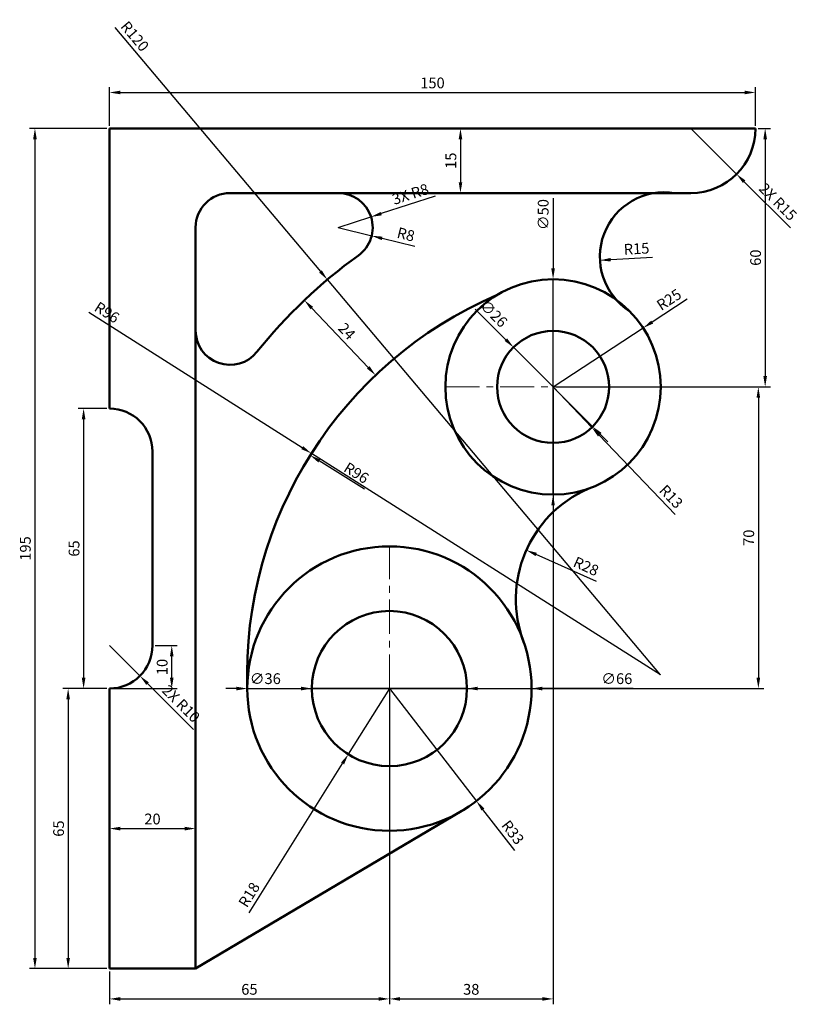
# Model space of a CAD drawing. Units: millimetres. Extents: x 2491 to 2672, y 889 to 1118.
import ezdxf

# ---------------------------------------------------------------- set-up
doc = ezdxf.new("R2010")
doc.units = ezdxf.units.MM
doc.linetypes.add('CENTER', pattern=[50.8, 31.75, -6.35, 6.35, -6.35])
for name, color, linetype, lineweight in [('M-CNTR', 4, 'CENTER', 18), ('M-DIMS', 2, 'Continuous', 25), ('M-OUTL', 7, 'Continuous', 50)]:
    doc.layers.add(name, color=color, linetype=linetype, lineweight=lineweight)
doc.styles.get("Standard").update_dxf_attribs({"font": 'arial.ttf'})
doc.dimstyles.new('ISO-25', dxfattribs={"dimtxt": 2.5, "dimasz": 2.5, "dimexe": 1.25, "dimexo": 0.625, "dimtad": 1, "dimtxsty": 'Standard', "dimcen": 2.5, "dimadec": 0, "dimazin": 0, "dimtfac": 1, "dimtmove": 0, "dimatfit": 3, "dimfxl": 1, "dimarcsym": 0})

# ---------------------------------------------------------------- blocks, each defined once
blk = doc.blocks.new('*D1')
at = {"layer": 'Defpoints', "color": 0, "transparency": 16777216}
for p in [(2511.93, 1092.34), (2494.64, 897.34), (2511.93, 897.34)]:
    blk.add_point(p, dxfattribs=at)
at = {"layer": 'M-DIMS', "color": 0, "lineweight": -2, "transparency": 16777216}
for p, q in [((2511.31, 1092.34), (2493.39, 1092.34)), ((2494.64, 1089.84), (2494.64, 899.84)), ((2511.31, 897.34), (2493.39, 897.34))]:
    blk.add_line(p, q, dxfattribs=at)
at = {"layer": 'M-DIMS', "color": 0, "transparency": 16777216}
for points in [[(2494.22, 1089.84), (2495.06, 1089.84), (2494.64, 1092.34)], [(2494.22, 899.84), (2495.06, 899.84), (2494.64, 897.34)]]:
    blk.add_solid(points, dxfattribs=at)
at = {"layer": 'M-DIMS', "color": 0, "transparency": 16777216, "insert": (2492.74, 994.84), "char_height": 2.5, "attachment_point": 5, "rotation": 90}
blk.add_mtext('195', dxfattribs=at)
blk = doc.blocks.new('*D2')
at = {"layer": 'Defpoints', "color": 0, "transparency": 16777216}
for p in [(2661.93, 1100.67), (2511.93, 1092.34), (2661.93, 1092.34)]:
    blk.add_point(p, dxfattribs=at)
at = {"layer": 'M-DIMS', "color": 0, "lineweight": -2, "transparency": 16777216}
for p, q in [((2511.93, 1092.96), (2511.93, 1101.92)), ((2661.93, 1092.96), (2661.93, 1101.92)), ((2514.43, 1100.67), (2659.43, 1100.67))]:
    blk.add_line(p, q, dxfattribs=at)
at = {"layer": 'M-DIMS', "color": 0, "transparency": 16777216}
for points in [[(2514.43, 1101.09), (2514.43, 1100.26), (2511.93, 1100.67)], [(2659.43, 1101.09), (2659.43, 1100.26), (2661.93, 1100.67)]]:
    blk.add_solid(points, dxfattribs=at)
at = {"layer": 'M-DIMS', "color": 0, "transparency": 16777216, "insert": (2586.93, 1102.57), "char_height": 2.5, "attachment_point": 5}
blk.add_mtext('150', dxfattribs=at)
blk = doc.blocks.new('*D3')
at = {"layer": 'Defpoints', "color": 0, "transparency": 16777216}
for p in [(2586.93, 1092.34), (2586.93, 1077.34), (2593.43, 1077.34)]:
    blk.add_point(p, dxfattribs=at)
at = {"layer": 'M-DIMS', "color": 0, "lineweight": -2, "transparency": 16777216}
for p, q in [((2587.56, 1092.34), (2594.68, 1092.34)), ((2593.43, 1089.84), (2593.43, 1079.84)), ((2587.56, 1077.34), (2594.68, 1077.34))]:
    blk.add_line(p, q, dxfattribs=at)
at = {"layer": 'M-DIMS', "color": 0, "transparency": 16777216}
for points in [[(2593.02, 1089.84), (2593.85, 1089.84), (2593.43, 1092.34)], [(2593.02, 1079.84), (2593.85, 1079.84), (2593.43, 1077.34)]]:
    blk.add_solid(points, dxfattribs=at)
at = {"layer": 'M-DIMS', "color": 0, "transparency": 16777216, "insert": (2591.53, 1084.84), "char_height": 2.5, "attachment_point": 5, "rotation": 90}
blk.add_mtext('15', dxfattribs=at)
blk = doc.blocks.new('*D4')
at = {"layer": 'Defpoints', "color": 0, "transparency": 16777216}
for p in [(2557.19, 1052.45), (2573.73, 1035.06), (2573.73, 1035.06)]:
    blk.add_point(p, dxfattribs=at)
at = {"layer": 'M-DIMS', "color": 0, "lineweight": -2, "transparency": 16777216}
for p, q in [((2557.65, 1052.89), (2558.1, 1053.32)), ((2558.92, 1050.64), (2572.01, 1036.87)), ((2574.18, 1035.49), (2574.64, 1035.92))]:
    blk.add_line(p, q, dxfattribs=at)
at = {"layer": 'M-DIMS', "color": 0, "transparency": 16777216}
for points in [[(2559.22, 1050.93), (2558.61, 1050.36), (2557.19, 1052.45)], [(2572.31, 1037.16), (2571.71, 1036.59), (2573.73, 1035.06)]]:
    blk.add_solid(points, dxfattribs=at)
at = {"layer": 'M-DIMS', "color": 0, "transparency": 16777216, "insert": (2566.82, 1045.05), "char_height": 2.5, "attachment_point": 5, "rotation": 313.5577}
blk.add_mtext('24', dxfattribs=at)
blk = doc.blocks.new('*D5')
at = {"layer": 'Defpoints', "color": 0, "transparency": 16777216}
for p in [(2661.93, 1092.34), (2614.93, 1032.34), (2664.17, 1032.34)]:
    blk.add_point(p, dxfattribs=at)
at = {"layer": 'M-DIMS', "color": 0, "lineweight": -2, "transparency": 16777216}
for p, q in [((2662.56, 1092.34), (2665.42, 1092.34)), ((2664.17, 1089.84), (2664.17, 1034.84)), ((2615.56, 1032.34), (2665.42, 1032.34))]:
    blk.add_line(p, q, dxfattribs=at)
at = {"layer": 'M-DIMS', "color": 0, "transparency": 16777216}
for points in [[(2663.76, 1089.84), (2664.59, 1089.84), (2664.17, 1092.34)], [(2663.76, 1034.84), (2664.59, 1034.84), (2664.17, 1032.34)]]:
    blk.add_solid(points, dxfattribs=at)
at = {"layer": 'M-DIMS', "color": 0, "transparency": 16777216, "insert": (2662.27, 1062.34), "char_height": 2.5, "attachment_point": 5, "rotation": 90}
blk.add_mtext('60', dxfattribs=at)
blk = doc.blocks.new('*D6')
at = {"layer": 'Defpoints', "color": 0, "transparency": 16777216}
for p in [(2614.93, 1032.34), (2576.93, 962.34), (2662.59, 962.34)]:
    blk.add_point(p, dxfattribs=at)
at = {"layer": 'M-DIMS', "color": 0, "lineweight": -2, "transparency": 16777216}
for p, q in [((2615.56, 1032.34), (2663.84, 1032.34)), ((2662.59, 1029.84), (2662.59, 964.84)), ((2577.56, 962.34), (2663.84, 962.34))]:
    blk.add_line(p, q, dxfattribs=at)
at = {"layer": 'M-DIMS', "color": 0, "transparency": 16777216}
for points in [[(2662.17, 1029.84), (2663, 1029.84), (2662.59, 1032.34)], [(2662.17, 964.84), (2663, 964.84), (2662.59, 962.34)]]:
    blk.add_solid(points, dxfattribs=at)
at = {"layer": 'M-DIMS', "color": 0, "transparency": 16777216, "insert": (2660.68, 997.34), "char_height": 2.5, "attachment_point": 5, "rotation": 90}
blk.add_mtext('70', dxfattribs=at)
blk = doc.blocks.new('*D7')
at = {"layer": 'Defpoints', "color": 0, "transparency": 16777216}
for p in [(2576.93, 962.34), (2511.93, 897.34), (2576.93, 890.31)]:
    blk.add_point(p, dxfattribs=at)
at = {"layer": 'M-DIMS', "color": 0, "lineweight": -2, "transparency": 16777216}
for p, q in [((2576.93, 961.71), (2576.93, 889.06)), ((2511.93, 896.71), (2511.93, 889.06)), ((2514.43, 890.31), (2574.43, 890.31))]:
    blk.add_line(p, q, dxfattribs=at)
at = {"layer": 'M-DIMS', "color": 0, "transparency": 16777216}
for points in [[(2514.43, 890.73), (2514.43, 889.89), (2511.93, 890.31)], [(2574.43, 890.73), (2574.43, 889.89), (2576.93, 890.31)]]:
    blk.add_solid(points, dxfattribs=at)
at = {"layer": 'M-DIMS', "color": 0, "transparency": 16777216, "insert": (2544.43, 892.21), "char_height": 2.5, "attachment_point": 5}
blk.add_mtext('65', dxfattribs=at)
blk = doc.blocks.new('*D8')
at = {"layer": 'Defpoints', "color": 0, "transparency": 16777216}
for p in [(2614.93, 1032.34), (2576.93, 962.34), (2614.93, 890.31)]:
    blk.add_point(p, dxfattribs=at)
at = {"layer": 'M-DIMS', "color": 0, "lineweight": -2, "transparency": 16777216}
for p, q in [((2614.93, 1031.71), (2614.93, 889.06)), ((2576.93, 961.71), (2576.93, 889.06)), ((2579.43, 890.31), (2612.43, 890.31))]:
    blk.add_line(p, q, dxfattribs=at)
at = {"layer": 'M-DIMS', "color": 0, "transparency": 16777216}
for points in [[(2579.43, 890.73), (2579.43, 889.89), (2576.93, 890.31)], [(2612.43, 890.73), (2612.43, 889.89), (2614.93, 890.31)]]:
    blk.add_solid(points, dxfattribs=at)
at = {"layer": 'M-DIMS', "color": 0, "transparency": 16777216, "insert": (2595.93, 892.21), "char_height": 2.5, "attachment_point": 5}
blk.add_mtext('38', dxfattribs=at)
blk = doc.blocks.new('*D9')
at = {"layer": 'Defpoints', "color": 0, "transparency": 16777216}
for p in [(2511.93, 1027.34), (2505.94, 962.34), (2511.93, 962.34)]:
    blk.add_point(p, dxfattribs=at)
at = {"layer": 'M-DIMS', "color": 0, "lineweight": -2, "transparency": 16777216}
for p, q in [((2511.31, 1027.34), (2504.69, 1027.34)), ((2505.94, 1024.84), (2505.94, 964.84)), ((2511.31, 962.34), (2504.69, 962.34))]:
    blk.add_line(p, q, dxfattribs=at)
at = {"layer": 'M-DIMS', "color": 0, "transparency": 16777216}
for points in [[(2505.52, 1024.84), (2506.36, 1024.84), (2505.94, 1027.34)], [(2505.52, 964.84), (2506.36, 964.84), (2505.94, 962.34)]]:
    blk.add_solid(points, dxfattribs=at)
at = {"layer": 'M-DIMS', "color": 0, "transparency": 16777216, "insert": (2504.04, 994.84), "char_height": 2.5, "attachment_point": 5, "rotation": 90}
blk.add_mtext('65', dxfattribs=at)
blk = doc.blocks.new('*D10')
at = {"layer": 'Defpoints', "color": 0, "transparency": 16777216}
for p in [(2511.93, 962.34), (2502.35, 897.34), (2511.93, 897.34)]:
    blk.add_point(p, dxfattribs=at)
at = {"layer": 'M-DIMS', "color": 0, "lineweight": -2, "transparency": 16777216}
for p, q in [((2511.31, 962.34), (2501.1, 962.34)), ((2502.35, 959.84), (2502.35, 899.84)), ((2511.31, 897.34), (2501.1, 897.34))]:
    blk.add_line(p, q, dxfattribs=at)
at = {"layer": 'M-DIMS', "color": 0, "transparency": 16777216}
for points in [[(2501.93, 959.84), (2502.77, 959.84), (2502.35, 962.34)], [(2501.93, 899.84), (2502.77, 899.84), (2502.35, 897.34)]]:
    blk.add_solid(points, dxfattribs=at)
at = {"layer": 'M-DIMS', "color": 0, "transparency": 16777216, "insert": (2500.45, 929.84), "char_height": 2.5, "attachment_point": 5, "rotation": 90}
blk.add_mtext('65', dxfattribs=at)
blk = doc.blocks.new('*D11')
at = {"layer": 'Defpoints', "color": 0, "transparency": 16777216}
for p in [(2625.82, 1061.73), (2640.8, 1062.54)]:
    blk.add_point(p, dxfattribs=at)
at = {"layer": 'M-DIMS', "color": 0, "lineweight": -2, "transparency": 16777216}
blk.add_line((2638.04, 1062.39), (2628.32, 1061.87), dxfattribs=at)
at = {"layer": 'M-DIMS', "color": 0, "transparency": 16777216}
blk.add_solid([(2628.29, 1062.28), (2628.34, 1061.45), (2625.82, 1061.73)], dxfattribs=at)
at = {"layer": 'M-DIMS', "color": 0, "transparency": 16777216, "insert": (2634.33, 1064.09), "char_height": 2.5, "attachment_point": 5, "rotation": 3.074}
blk.add_mtext('R15', dxfattribs=at)
blk = doc.blocks.new('*D12')
at = {"layer": 'Defpoints', "color": 0, "transparency": 16777216}
for p in [(2635.85, 1046.03), (2614.93, 1032.34)]:
    blk.add_point(p, dxfattribs=at)
at = {"layer": 'M-DIMS', "color": 0, "lineweight": -2, "transparency": 16777216}
for p, q in [((2646.1, 1052.74), (2637.94, 1047.4)), ((2614.93, 1032.34), (2635.85, 1046.03))]:
    blk.add_line(p, q, dxfattribs=at)
at = {"layer": 'M-DIMS', "color": 0, "transparency": 16777216}
blk.add_solid([(2637.72, 1047.75), (2638.17, 1047.05), (2635.85, 1046.03)], dxfattribs=at)
at = {"layer": 'M-DIMS', "color": 0, "transparency": 16777216, "insert": (2642.02, 1052.34), "char_height": 2.5, "attachment_point": 5, "rotation": 33.2069}
blk.add_mtext('R25', dxfattribs=at)
blk = doc.blocks.new('*D13')
at = {"layer": 'Defpoints', "color": 0, "transparency": 16777216}
for p in [(2614.93, 1032.34), (2623.92, 1022.94)]:
    blk.add_point(p, dxfattribs=at)
at = {"layer": 'M-DIMS', "color": 0, "lineweight": -2, "transparency": 16777216}
for p, q in [((2614.93, 1032.34), (2623.92, 1022.94)), ((2643.24, 1002.73), (2625.65, 1021.14))]:
    blk.add_line(p, q, dxfattribs=at)
at = {"layer": 'M-DIMS', "color": 0, "transparency": 16777216}
blk.add_solid([(2625.95, 1021.42), (2625.35, 1020.85), (2623.92, 1022.94)], dxfattribs=at)
at = {"layer": 'M-DIMS', "color": 0, "transparency": 16777216, "insert": (2642.12, 1006.66), "char_height": 2.5, "attachment_point": 5, "rotation": 313.7163}
blk.add_mtext('R13', dxfattribs=at)
blk = doc.blocks.new('*D14')
at = {"layer": 'Defpoints', "color": 0, "transparency": 16777216}
for p in [(2608.73, 994.47), (2634.3, 983.05)]:
    blk.add_point(p, dxfattribs=at)
at = {"layer": 'M-DIMS', "color": 0, "lineweight": -2, "transparency": 16777216}
blk.add_line((2624.99, 987.21), (2611.01, 993.45), dxfattribs=at)
at = {"layer": 'M-DIMS', "color": 0, "transparency": 16777216}
blk.add_solid([(2611.18, 993.83), (2610.85, 993.07), (2608.73, 994.47)], dxfattribs=at)
at = {"layer": 'M-DIMS', "color": 0, "transparency": 16777216, "insert": (2622.47, 990.42), "char_height": 2.5, "attachment_point": 5, "rotation": 335.934}
blk.add_mtext('R28', dxfattribs=at)
blk = doc.blocks.new('*D15')
at = {"layer": 'Defpoints', "color": 0, "transparency": 16777216}
for p in [(2558.54, 1016.48), (2639.88, 965.49)]:
    blk.add_point(p, dxfattribs=at)
at = {"layer": 'M-DIMS', "color": 0, "lineweight": -2, "transparency": 16777216}
blk.add_line((2571.15, 1008.58), (2560.66, 1015.16), dxfattribs=at)
at = {"layer": 'M-DIMS', "color": 0, "transparency": 16777216}
blk.add_solid([(2560.88, 1015.51), (2560.44, 1014.8), (2558.54, 1016.48)], dxfattribs=at)
at = {"layer": 'M-DIMS', "color": 0, "transparency": 16777216, "insert": (2569.1, 1012.11), "char_height": 2.5, "attachment_point": 5, "rotation": 327.9171}
blk.add_mtext('R96', dxfattribs=at)
blk = doc.blocks.new('*D16')
at = {"layer": 'Defpoints', "color": 0, "transparency": 16777216}
for p in [(2576.93, 962.34), (2567.39, 947.08)]:
    blk.add_point(p, dxfattribs=at)
at = {"layer": 'M-DIMS', "color": 0, "lineweight": -2, "transparency": 16777216}
for p, q in [((2576.93, 962.34), (2567.39, 947.08)), ((2544.34, 910.25), (2566.06, 944.96))]:
    blk.add_line(p, q, dxfattribs=at)
at = {"layer": 'M-DIMS', "color": 0, "transparency": 16777216}
blk.add_solid([(2565.71, 945.18), (2566.41, 944.74), (2567.39, 947.08)], dxfattribs=at)
at = {"layer": 'M-DIMS', "color": 0, "transparency": 16777216, "insert": (2544.64, 914.32), "char_height": 2.5, "attachment_point": 5, "rotation": 57.9594}
blk.add_mtext('R18', dxfattribs=at)
blk = doc.blocks.new('*D17')
at = {"layer": 'Defpoints', "color": 0, "transparency": 16777216}
for p in [(2576.93, 962.34), (2597.13, 936.24)]:
    blk.add_point(p, dxfattribs=at)
at = {"layer": 'M-DIMS', "color": 0, "lineweight": -2, "transparency": 16777216}
for p, q in [((2576.93, 962.34), (2597.13, 936.24)), ((2606.03, 924.74), (2598.66, 934.26))]:
    blk.add_line(p, q, dxfattribs=at)
at = {"layer": 'M-DIMS', "color": 0, "transparency": 16777216}
blk.add_solid([(2598.99, 934.52), (2598.33, 934.01), (2597.13, 936.24)], dxfattribs=at)
at = {"layer": 'M-DIMS', "color": 0, "transparency": 16777216, "insert": (2605.33, 928.76), "char_height": 2.5, "attachment_point": 5, "rotation": 307.7377}
blk.add_mtext('R33', dxfattribs=at)
blk = doc.blocks.new('*D18')
at = {"layer": 'Defpoints', "color": 0, "transparency": 16777216}
for p in [(2565.05, 1069.34), (2572.82, 1067.42)]:
    blk.add_point(p, dxfattribs=at)
at = {"layer": 'M-DIMS', "color": 0, "lineweight": -2, "transparency": 16777216}
for p, q in [((2565.05, 1069.34), (2572.82, 1067.42)), ((2582.8, 1064.95), (2575.24, 1066.82))]:
    blk.add_line(p, q, dxfattribs=at)
at = {"layer": 'M-DIMS', "color": 0, "transparency": 16777216}
blk.add_solid([(2575.34, 1067.22), (2575.14, 1066.41), (2572.82, 1067.42)], dxfattribs=at)
at = {"layer": 'M-DIMS', "color": 0, "transparency": 16777216, "insert": (2580.69, 1067.43), "char_height": 2.5, "attachment_point": 5, "rotation": 346.101}
blk.add_mtext('R8', dxfattribs=at)
blk = doc.blocks.new('*D19')
at = {"layer": 'Defpoints', "color": 0, "transparency": 16777216}
for p in [(2511.93, 929.84), (2531.93, 929.84), (2531.93, 929.84)]:
    blk.add_point(p, dxfattribs=at)
at = {"layer": 'M-DIMS', "color": 0, "lineweight": -2, "transparency": 16777216}
for p, q in [((2511.93, 930.46), (2511.93, 931.09)), ((2531.93, 930.46), (2531.93, 931.09)), ((2514.43, 929.84), (2529.43, 929.84))]:
    blk.add_line(p, q, dxfattribs=at)
at = {"layer": 'M-DIMS', "color": 0, "transparency": 16777216}
for points in [[(2514.43, 930.26), (2514.43, 929.42), (2511.93, 929.84)], [(2529.43, 930.26), (2529.43, 929.42), (2531.93, 929.84)]]:
    blk.add_solid(points, dxfattribs=at)
at = {"layer": 'M-DIMS', "color": 0, "transparency": 16777216, "insert": (2521.93, 931.74), "char_height": 2.5, "attachment_point": 5}
blk.add_mtext('20', dxfattribs=at)
blk = doc.blocks.new('*D20')
at = {"layer": 'Defpoints', "color": 0, "transparency": 16777216}
for p in [(2521.93, 972.34), (2526.4, 972.34), (2511.93, 962.34)]:
    blk.add_point(p, dxfattribs=at)
at = {"layer": 'M-DIMS', "color": 0, "lineweight": -2, "transparency": 16777216}
for p, q in [((2522.56, 972.34), (2527.65, 972.34)), ((2526.4, 964.84), (2526.4, 969.84)), ((2512.56, 962.34), (2527.65, 962.34))]:
    blk.add_line(p, q, dxfattribs=at)
at = {"layer": 'M-DIMS', "color": 0, "transparency": 16777216}
for points in [[(2525.99, 969.84), (2526.82, 969.84), (2526.4, 972.34)], [(2525.99, 964.84), (2526.82, 964.84), (2526.4, 962.34)]]:
    blk.add_solid(points, dxfattribs=at)
at = {"layer": 'M-DIMS', "color": 0, "transparency": 16777216, "insert": (2524.5, 967.34), "char_height": 2.5, "attachment_point": 5, "rotation": 90}
blk.add_mtext('10', dxfattribs=at)
blk = doc.blocks.new('*D21')
at = {"layer": 'Defpoints', "color": 0, "transparency": 16777216}
for p in [(2543.93, 962.34), (2609.93, 962.34)]:
    blk.add_point(p, dxfattribs=at)
at = {"layer": 'M-DIMS', "color": 0, "lineweight": -2, "transparency": 16777216}
for p, q in [((2541.43, 962.34), (2538.93, 962.34)), ((2543.93, 962.34), (2609.93, 962.34)), ((2633.51, 962.34), (2612.43, 962.34))]:
    blk.add_line(p, q, dxfattribs=at)
at = {"layer": 'M-DIMS', "color": 0, "transparency": 16777216}
for points in [[(2541.43, 962.76), (2541.43, 961.92), (2543.93, 962.34)], [(2612.43, 962.76), (2612.43, 961.92), (2609.93, 962.34)]]:
    blk.add_solid(points, dxfattribs=at)
at = {"layer": 'M-DIMS', "color": 0, "transparency": 16777216, "insert": (2629.73, 964.31), "char_height": 2.5, "attachment_point": 5, "rotation": 0.0005}
blk.add_mtext('∅66', dxfattribs=at)
blk = doc.blocks.new('*D22')
at = {"layer": 'Defpoints', "color": 0, "transparency": 16777216}
for p in [(2614.93, 1057.34), (2614.93, 1007.34)]:
    blk.add_point(p, dxfattribs=at)
at = {"layer": 'M-DIMS', "color": 0, "lineweight": -2, "transparency": 16777216}
for p, q in [((2614.93, 1076.11), (2614.93, 1059.84)), ((2614.93, 1007.34), (2614.93, 1057.34)), ((2614.93, 1004.84), (2614.93, 1002.34))]:
    blk.add_line(p, q, dxfattribs=at)
at = {"layer": 'M-DIMS', "color": 0, "transparency": 16777216}
for points in [[(2614.52, 1059.84), (2615.35, 1059.84), (2614.93, 1057.34)], [(2614.52, 1004.84), (2615.35, 1004.84), (2614.93, 1007.34)]]:
    blk.add_solid(points, dxfattribs=at)
at = {"layer": 'M-DIMS', "color": 0, "transparency": 16777216, "insert": (2612.96, 1072.34), "char_height": 2.5, "attachment_point": 5, "rotation": 89.9998}
blk.add_mtext('∅50', dxfattribs=at)
blk = doc.blocks.new('*D23')
at = {"layer": 'Defpoints', "color": 0, "transparency": 16777216}
for p in [(2558.93, 962.34), (2594.93, 962.34)]:
    blk.add_point(p, dxfattribs=at)
at = {"layer": 'M-DIMS', "color": 0, "lineweight": -2, "transparency": 16777216}
for p, q in [((2544.36, 962.34), (2556.43, 962.34)), ((2594.93, 962.34), (2558.93, 962.34)), ((2597.43, 962.34), (2599.93, 962.34))]:
    blk.add_line(p, q, dxfattribs=at)
at = {"layer": 'M-DIMS', "color": 0, "transparency": 16777216}
for points in [[(2556.43, 962.76), (2556.43, 961.92), (2558.93, 962.34)], [(2597.43, 962.76), (2597.43, 961.92), (2594.93, 962.34)]]:
    blk.add_solid(points, dxfattribs=at)
at = {"layer": 'M-DIMS', "color": 0, "transparency": 16777216, "insert": (2548.13, 964.31), "char_height": 2.5, "attachment_point": 5, "rotation": 359.9992}
blk.add_mtext('∅36', dxfattribs=at)
blk = doc.blocks.new('*D24')
at = {"layer": 'Defpoints', "color": 0, "transparency": 16777216}
for p in [(2605.75, 1041.53), (2624.12, 1023.14)]:
    blk.add_point(p, dxfattribs=at)
at = {"layer": 'M-DIMS', "color": 0, "lineweight": -2, "transparency": 16777216}
for p, q in [((2596.87, 1050.41), (2603.98, 1043.3)), ((2624.12, 1023.14), (2605.75, 1041.53)), ((2625.89, 1021.37), (2627.66, 1019.61))]:
    blk.add_line(p, q, dxfattribs=at)
at = {"layer": 'M-DIMS', "color": 0, "transparency": 16777216}
for points in [[(2604.27, 1043.6), (2603.68, 1043.01), (2605.75, 1041.53)], [(2626.19, 1021.67), (2625.6, 1021.08), (2624.12, 1023.14)]]:
    blk.add_solid(points, dxfattribs=at)
at = {"layer": 'M-DIMS', "color": 0, "transparency": 16777216, "insert": (2600.94, 1049.13), "char_height": 2.5, "attachment_point": 5, "rotation": 314.9801}
blk.add_mtext('∅26', dxfattribs=at)
blk = doc.blocks.new('*D25')
at = {"layer": 'Defpoints', "color": 0, "transparency": 16777216}
for p in [(2562.54, 1057.24), (2639.88, 965.49)]:
    blk.add_point(p, dxfattribs=at)
at = {"layer": 'M-DIMS', "color": 0, "lineweight": -2, "transparency": 16777216}
for p, q in [((2513.18, 1115.79), (2560.92, 1059.15)), ((2639.88, 965.49), (2562.54, 1057.24))]:
    blk.add_line(p, q, dxfattribs=at)
at = {"layer": 'M-DIMS', "color": 0, "transparency": 16777216}
blk.add_solid([(2561.24, 1059.42), (2560.61, 1058.88), (2562.54, 1057.24)], dxfattribs=at)
at = {"layer": 'M-DIMS', "color": 0, "transparency": 16777216, "insert": (2517.58, 1113.51), "char_height": 2.5, "attachment_point": 5, "rotation": 310.1329}
blk.add_mtext('R120', dxfattribs=at)
blk = doc.blocks.new('*D26')
at = {"layer": 'Defpoints', "color": 0, "transparency": 16777216}
for p in [(2558.81, 1016.91), (2639.88, 965.49)]:
    blk.add_point(p, dxfattribs=at)
at = {"layer": 'M-DIMS', "color": 0, "lineweight": -2, "transparency": 16777216}
for p, q in [((2507.12, 1049.69), (2556.7, 1018.25)), ((2639.88, 965.49), (2558.81, 1016.91))]:
    blk.add_line(p, q, dxfattribs=at)
at = {"layer": 'M-DIMS', "color": 0, "transparency": 16777216}
blk.add_solid([(2556.92, 1018.6), (2556.48, 1017.9), (2558.81, 1016.91)], dxfattribs=at)
at = {"layer": 'M-DIMS', "color": 0, "transparency": 16777216, "insert": (2511.19, 1049.36), "char_height": 2.5, "attachment_point": 5, "rotation": 327.6168}
blk.add_mtext('R96', dxfattribs=at)
blk = doc.blocks.new('*D27')
at = {"layer": 'Defpoints', "color": 0, "transparency": 16777216}
for p in [(2646.93, 1092.34), (2657.54, 1081.73)]:
    blk.add_point(p, dxfattribs=at)
at = {"layer": 'M-DIMS', "color": 0, "lineweight": -2, "transparency": 16777216}
for p, q in [((2646.93, 1092.34), (2657.54, 1081.73)), ((2670.03, 1069.25), (2659.31, 1079.96))]:
    blk.add_line(p, q, dxfattribs=at)
at = {"layer": 'M-DIMS', "color": 0, "transparency": 16777216}
blk.add_solid([(2659.6, 1080.26), (2659.01, 1079.67), (2657.54, 1081.73)], dxfattribs=at)
at = {"layer": 'M-DIMS', "color": 0, "transparency": 16777216, "insert": (2666.9, 1075.07), "char_height": 2.5, "attachment_point": 5, "rotation": 314.9983}
blk.add_mtext('2X R15', dxfattribs=at)
blk = doc.blocks.new('*D28')
at = {"layer": 'Defpoints', "color": 0, "transparency": 16777216}
for p in [(2511.93, 972.34), (2519.01, 965.27)]:
    blk.add_point(p, dxfattribs=at)
at = {"layer": 'M-DIMS', "color": 0, "lineweight": -2, "transparency": 16777216}
for p, q in [((2511.93, 972.34), (2519.01, 965.27)), ((2531.47, 952.8), (2520.77, 963.5))]:
    blk.add_line(p, q, dxfattribs=at)
at = {"layer": 'M-DIMS', "color": 0, "transparency": 16777216}
blk.add_solid([(2521.07, 963.79), (2520.48, 963.21), (2519.01, 965.27)], dxfattribs=at)
at = {"layer": 'M-DIMS', "color": 0, "transparency": 16777216, "insert": (2528.35, 958.61), "char_height": 2.5, "attachment_point": 5, "rotation": 315.0015}
blk.add_mtext('2X R10', dxfattribs=at)
blk = doc.blocks.new('*D29')
at = {"layer": 'Defpoints', "color": 0, "transparency": 16777216}
for p in [(2572.66, 1071.8), (2565.05, 1069.34)]:
    blk.add_point(p, dxfattribs=at)
at = {"layer": 'M-DIMS', "color": 0, "lineweight": -2, "transparency": 16777216}
for p, q in [((2587.56, 1076.6), (2575.04, 1072.56)), ((2565.05, 1069.34), (2572.66, 1071.8))]:
    blk.add_line(p, q, dxfattribs=at)
at = {"layer": 'M-DIMS', "color": 0, "transparency": 16777216}
blk.add_solid([(2574.91, 1072.96), (2575.17, 1072.17), (2572.66, 1071.8)], dxfattribs=at)
at = {"layer": 'M-DIMS', "color": 0, "transparency": 16777216, "insert": (2581.91, 1076.78), "char_height": 2.5, "attachment_point": 5, "rotation": 17.8873}
blk.add_mtext('3X R8', dxfattribs=at)

msp = doc.modelspace()

# ---------------------------------------------------------------- linework, layer by layer
at = {"layer": 'M-CNTR', "ltscale": 0.25}
for p, q in [((2614.935, 1057.339), (2614.935, 1032.339)), ((2589.935, 1032.339), (2639.935, 1032.339)), ((2614.935, 1007.339), (2614.935, 1032.339)), ((2576.935, 962.339), (2576.935, 995.339)), ((2576.935, 962.339), (2543.935, 962.339)), ((2576.935, 929.339), (2576.935, 962.339)), ((2576.935, 962.339), (2614.935, 962.339))]:
    msp.add_line(p, q, dxfattribs=at)
at = {"layer": 'M-OUTL'}
for p, q in [((2511.935, 1092.339), (2661.935, 1092.339)), ((2511.935, 1027.339), (2511.935, 1092.339)), ((2539.935, 1077.339), (2646.935, 1077.339)), ((2531.935, 897.339), (2531.935, 1069.339)), ((2521.935, 972.339), (2521.935, 1017.339)), ((2511.935, 897.339), (2511.935, 962.339)), ((2531.935, 897.339), (2593.75, 933.944)), ((2511.935, 897.339), (2531.935, 897.339))]:
    msp.add_line(p, q, dxfattribs=at)
for centre, radius in [((2614.935, 1032.339), 25), ((2614.935, 1032.339), 13), ((2576.935, 962.339), 33), ((2576.935, 962.339), 18)]:
    msp.add_circle(centre, radius, dxfattribs=at)
for centre, radius, start, end in [((2646.935, 1092.339), 15, 270, 0), ((2539.935, 1069.339), 8, 90, 180), ((2565.049, 1069.339), 8, 305.77743, 90), ((2640.798, 1062.537), 15, 80.67882, 237.54063), ((2639.883, 965.493), 120, 125.77743, 141.33801), ((2639.883, 965.493), 96, 113.35083, 181.88295), ((2539.935, 1045.458), 8, 180, 321.33801), ((2511.935, 1017.339), 10, 0, 90), ((2634.298, 983.051), 28, 113.68657, 201.06903), ((2511.935, 972.339), 10, 270, 0)]:
    msp.add_arc(centre, radius, start, end, dxfattribs=at)

# ---------------------------------------------------------------- dimensions: what is measured, and where the dimension line sits
at = {"layer": 'M-DIMS'}
for center, mpoint, override, picture, middle in [((2639.883, 965.493), (2562.536, 1057.239), {"dimdec": 0, "dimlfac": 1, "dimrnd": 0, "dimzin": 0, "dimdsep": 46, "dimlunit": 2}, '*D25', (2516.127, 1112.287)), ((2640.798, 1062.537), (2625.82, 1061.732), {"dimclrd": 0, "dimclre": 0, "dimclrt": 0}, '*D11', (2634.429, 1062.195)), ((2639.883, 965.493), (2558.812, 1016.909), {"dimdec": 0, "dimlfac": 1, "dimrnd": 0, "dimzin": 0, "dimdsep": 46, "dimlunit": 2}, '*D26', (2510.17, 1047.758)), ((2614.935, 1032.339), (2623.919, 1022.943), {"dimclrd": 0, "dimclre": 0, "dimclrt": 0}, '*D13', (2640.748, 1005.342)), ((2639.883, 965.493), (2558.544, 1016.483), {"dimclrd": 0, "dimclre": 0, "dimclrt": 0}, '*D15', (2568.091, 1010.499)), ((2634.298, 983.051), (2608.732, 994.469), {"dimclrd": 0, "dimclre": 0, "dimclrt": 0}, '*D14', (2621.691, 988.682)), ((2576.935, 962.339), (2567.386, 947.081), {"dimclrd": 0, "dimclre": 0, "dimclrt": 0}, '*D16', (2546.254, 913.316)), ((2576.935, 962.339), (2597.132, 936.242), {"dimclrd": 0, "dimclre": 0, "dimclrt": 0}, '*D17', (2603.824, 927.596))]:
    dim = msp.add_radius_dim(center=center, mpoint=mpoint, dimstyle='ISO-25', override=override, dxfattribs=at)
    dim.commit()
    dim.dimension.update_dxf_attribs({"geometry": picture, "text_midpoint": middle, "dimtype": 164})
for base, p1, p2, picture, middle in [((2661.935, 1100.672), (2511.935, 1092.339), (2661.935, 1092.339), '*D2', (2586.935, 1102.573)), ((2614.935, 890.309), (2576.935, 962.339), (2614.935, 1032.339), '*D8', (2595.935, 892.211)), ((2576.935, 890.309), (2511.935, 897.339), (2576.935, 962.339), '*D7', (2544.435, 892.211)), ((2531.935, 929.839), (2511.935, 929.839), (2531.935, 929.839), '*D19', (2521.935, 931.74))]:
    dim = msp.add_linear_dim(base=base, p1=p1, p2=p2, dimstyle='ISO-25', override={"dimclrd": 0, "dimclre": 0, "dimclrt": 0}, dxfattribs=at)
    dim.commit()
    dim.dimension.update_dxf_attribs({"geometry": picture, "text_midpoint": middle})
for base, p1, p2, picture, middle in [((2494.639, 897.339), (2511.935, 1092.339), (2511.935, 897.339), '*D1', (2492.738, 994.839)), ((2593.435, 1077.339), (2586.935, 1092.339), (2586.935, 1077.339), '*D3', (2591.533, 1084.839)), ((2664.173, 1032.339), (2661.935, 1092.339), (2614.935, 1032.339), '*D5', (2662.272, 1062.339)), ((2662.585, 962.339), (2614.935, 1032.339), (2576.935, 962.339), '*D6', (2660.684, 997.339)), ((2505.94, 962.339), (2511.935, 1027.339), (2511.935, 962.339), '*D9', (2504.039, 994.839)), ((2526.402, 972.339), (2511.935, 962.339), (2521.935, 972.339), '*D20', (2524.5, 967.339)), ((2502.349, 897.339), (2511.935, 962.339), (2511.935, 897.339), '*D10', (2500.448, 929.839))]:
    dim = msp.add_linear_dim(base=base, p1=p1, p2=p2, angle=90, dimstyle='ISO-25', override={"dimclrd": 0, "dimclre": 0, "dimclrt": 0}, dxfattribs=at)
    dim.commit()
    dim.dimension.update_dxf_attribs({"geometry": picture, "text_midpoint": middle})
for center, mpoint, text, picture, middle in [((2646.935, 1092.339), (2657.541, 1081.732), '2X <>', '*D27', (2666.896, 1075.066)), ((2565.049, 1069.339), (2572.663, 1071.796), '3X <>', '*D29', (2581.907, 1076.779)), ((2511.935, 972.339), (2519.006, 965.268), '2X <>', '*D28', (2528.352, 958.612))]:
    dim = msp.add_radius_dim(center=center, mpoint=mpoint, text=text, dimstyle='ISO-25', override={"dimdec": 0, "dimlfac": 1, "dimrnd": 0, "dimzin": 0, "dimdsep": 46, "dimlunit": 2}, dxfattribs=at)
    dim.commit()
    dim.dimension.update_dxf_attribs({"geometry": picture, "text_midpoint": middle})
for p1, p2, picture, middle in [((2614.935, 1007.339), (2614.935, 1057.339), '*D22', (2614.935, 1072.339)), ((2543.935, 962.338), (2609.935, 962.339), '*D21', (2629.735, 962.339)), ((2594.935, 962.338), (2558.935, 962.339), '*D23', (2548.135, 962.339))]:
    dim = msp.add_diameter_dim_2p(p1=p1, p2=p2, dimstyle='ISO-25', override={"dimdec": 0, "dimlfac": 1, "dimrnd": 0, "dimzin": 0, "dimdsep": 46, "dimlunit": 2}, dxfattribs=at)
    dim.commit()
    dim.dimension.update_dxf_attribs({"geometry": picture, "text_midpoint": middle, "dimtype": 163})
for center, mpoint, picture, middle in [((2565.049, 1069.339), (2572.815, 1067.417), '*D18', (2580.691, 1067.427)), ((2614.935, 1032.339), (2635.852, 1046.03), '*D12', (2642.024, 1052.343))]:
    dim = msp.add_radius_dim(center=center, mpoint=mpoint, dimstyle='ISO-25', override={"dimclrd": 0, "dimclre": 0, "dimclrt": 0}, dxfattribs=at)
    dim.commit()
    dim.dimension.update_dxf_attribs({"geometry": picture, "text_midpoint": middle})
dim = msp.add_aligned_dim(p1=(2557.193, 1052.455), p2=(2573.731, 1035.062), distance=0, dimstyle='ISO-25', override={"dimclrd": 0, "dimclre": 0, "dimclrt": 0}, dxfattribs=at)
dim.commit()
dim.dimension.update_dxf_attribs({"geometry": '*D4', "text_midpoint": (2566.824, 1045.054)})
dim = msp.add_diameter_dim_2p(p1=(2624.124, 1023.143), p2=(2605.746, 1041.534), dimstyle='ISO-25', override={"dimdec": 0, "dimlfac": 1, "dimrnd": 0, "dimzin": 0, "dimdsep": 46, "dimlunit": 2}, dxfattribs=at)
dim.commit()
dim.dimension.update_dxf_attribs({"geometry": '*D24', "text_midpoint": (2599.543, 1047.741)})

doc.saveas('drawing.dxf')
